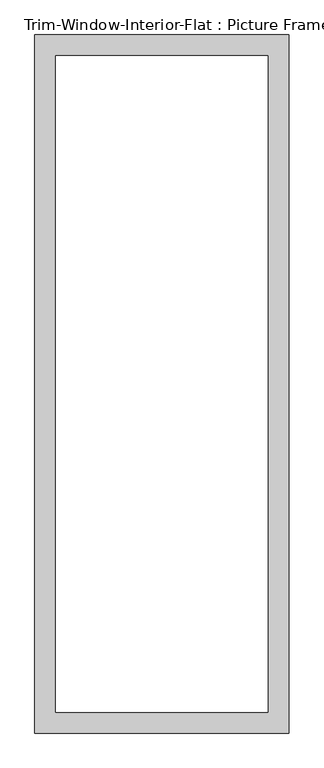
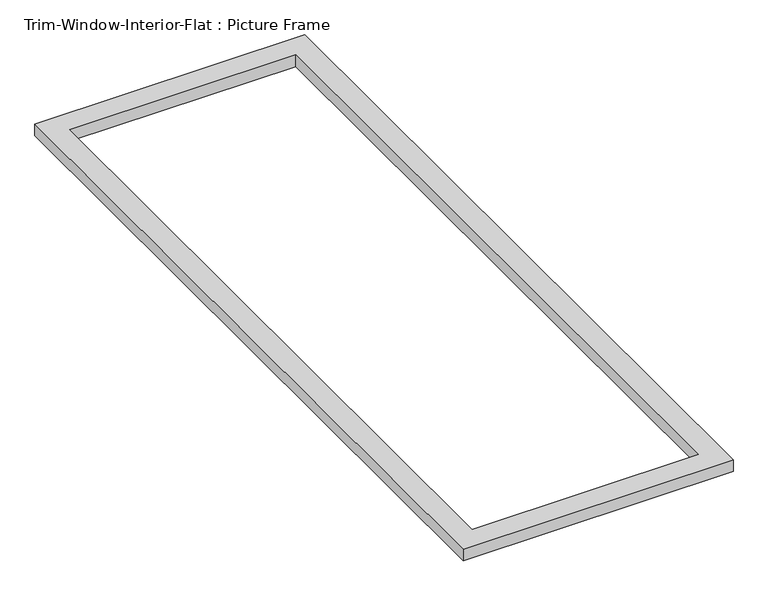
"""IFC4 building model written with IfcOpenShell, lengths in millimetres: proxy geometry, Trim-Window-Interior-Flat : Picture Frame."""

from ifc_helpers import new_model, si_unit, origin, origin_with_axes, place, context, project, spatial, polyline, outline, extrude, source, transform, mapped, element, save


def trim_window_interior_flat_picture_frame_6ac783dc(model_context):
    return source(origin(), model_context, "Body", "SweptSolid", [
        extrude(outline(polyline([(349.25, 44.45), (349.25, -1873.25), (-349.25, -1873.25), (-349.25, 44.45), (349.25, 44.45)]), holes=[polyline([(292.1, -12.7), (-292.1, -12.7), (-292.1, -1816.1), (292.1, -1816.1), (292.1, -12.7)])]), origin_with_axes(), (0.0, 0.0, 1.0), 31.75),
    ])


if __name__ == "__main__":
    model = new_model("IFC4")
    model_context = context("Model", 3, world=origin())
    ifc_project = project(units=[si_unit("LENGTHUNIT", "METRE", prefix="MILLI")], contexts=[model_context])
    site = spatial("IfcSite", under=ifc_project)
    building = spatial("IfcBuilding", under=site)
    placement = place(None, origin())
    trim_window_interior_flat_picture_frame_shape = trim_window_interior_flat_picture_frame_6ac783dc(model_context)
    element("IfcBuildingElementProxy", 1, Name="Trim-Window-Interior-Flat : Picture Frame", ObjectType="Trim-Window-Interior-Flat : Picture Frame", at=placement, inside=building, context=model_context, shape_type="MappedRepresentation", body=[
        mapped(trim_window_interior_flat_picture_frame_shape, transform((0.0, 0.0, 0.0), x_axis=(1.0, 0.0, 0.0), y_axis=(0.0, 1.0, 0.0), z_axis=(0.0, 0.0, 1.0))),
    ])
    save(model, "model.ifc")

# Revit data of these elements
# Type "Trim-Window-Interior-Flat : Picture Frame"
#   Trim Thickness_Picture Frame = 0' - 1 1/4"
#   Trim Width = 0' - 2 1/4"
#   Trim Thickness_with Sill = 0' - 0 3/4"
#   Sill Thickness = 0' - 1 1/4"
#   Opening Width [instance default] = 2' - 0"
#   Opening Height [instance default] = 3' - 0"
#   Default Elevation = 4' - 0"
#   Sill = no
#   Picture Frame = yes
#   Trim Material [instance default] = none
# Element 1 (IfcBuildingElementProxy, "Trim-Window-Interior-Flat : Picture Frame")
#   Opening Height = 6' - 0"
#   Trim Material = Wood - Stained
#   Materials on its faces: "Wood - Stained"
# Materials
#   "Wood - Stained": class "Wood", colour RGB 224 178 126, transparency 0, Cost = 0
